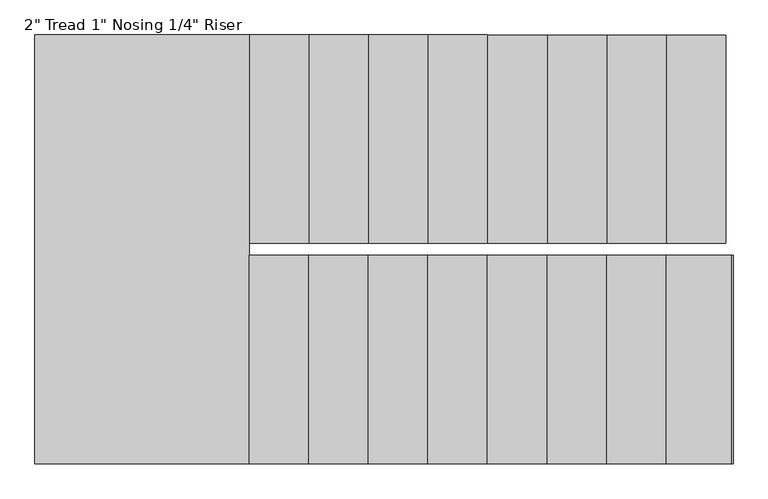
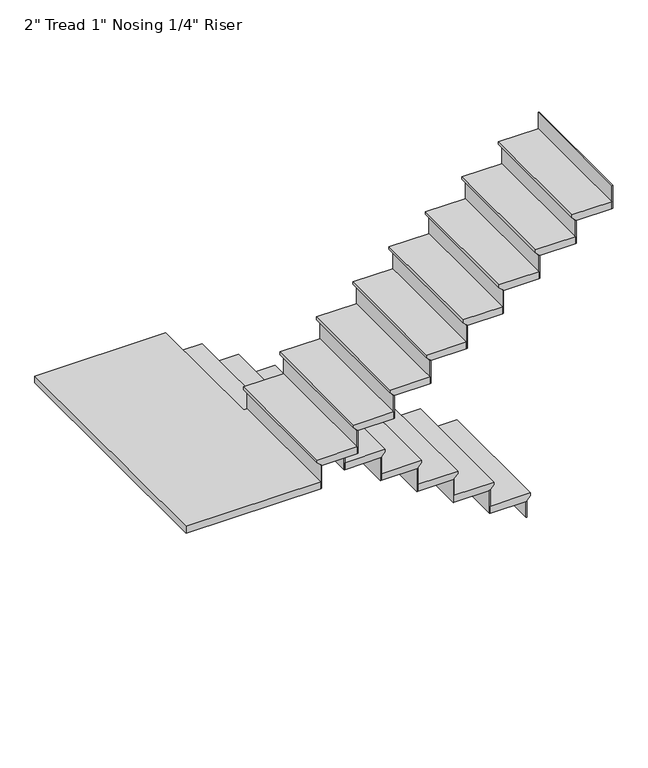
"""IFC4 building model written with IfcOpenShell, lengths in millimetres: stair flight geometry."""

from ifc_helpers import new_model, si_unit, origin, place, context, project, spatial, faceted_brep, source, transform, mapped, element, save


def stair_flight_f55dda53(model_context):
    return source(origin(), model_context, "Body", "Brep", [
        faceted_brep([(-2748.0012202, 5930.6309003, 15390.2833333), (-2748.0012202, 5930.6309003, 15409.3333333), (-2748.0012202, 5041.6309003, 15409.3333333), (-2748.0012202, 5041.6309003, 15390.2833333), (-2773.4012202, 5930.6309003, 15364.8833333), (-2773.4012202, 5041.6309003, 15364.8833333), (-3027.4012202, 5930.6309003, 15409.3333333), (-3027.4012202, 5041.6309003, 15409.3333333), (-2773.4012202, 5041.6309003, 15358.5333333), (-3027.4012202, 5041.6309003, 15358.5333333), (-3027.4012202, 5930.6309003, 15358.5333333), (-2773.4012202, 5930.6309003, 15358.5333333)], [[[0, 1, 2, 3]], [[4, 0, 3, 5]], [[2, 1, 6, 7]], [[8, 9, 10, 11]], [[2, 7, 9, 8, 5, 3]], [[8, 11, 4, 5]], [[6, 1, 0, 4, 11, 10]], [[7, 6, 10, 9]]]),
        faceted_brep([(-2773.4012202, 5930.6309003, 15358.5333333), (-2773.4012202, 5930.6309003, 15240.0), (-2779.7512202, 5930.6309003, 15240.0), (-2779.7512202, 5930.6309003, 15358.5333333), (-2773.4012202, 5041.6309003, 15358.5333333), (-2779.7512202, 5041.6309003, 15358.5333333), (-2779.7512202, 5041.6309003, 15240.0), (-2773.4012202, 5041.6309003, 15240.0)], [[[0, 1, 2, 3]], [[4, 5, 6, 7]], [[1, 0, 4, 7]], [[2, 1, 7, 6]], [[3, 2, 6, 5]], [[0, 3, 5, 4]]]),
        faceted_brep([(-3027.4012202, 5930.6309003, 15527.8666667), (-3027.4012202, 5930.6309003, 15358.5333333), (-3033.7512202, 5930.6309003, 15358.5333333), (-3033.7512202, 5930.6309003, 15527.8666667), (-3027.4012202, 5041.6309003, 15527.8666667), (-3033.7512202, 5041.6309003, 15527.8666667), (-3033.7512202, 5041.6309003, 15358.5333333), (-3027.4012202, 5041.6309003, 15358.5333333)], [[[0, 1, 2, 3]], [[4, 5, 6, 7]], [[1, 0, 4, 7]], [[2, 1, 7, 6]], [[3, 2, 6, 5]], [[0, 3, 5, 4]]]),
        faceted_brep([(-3002.0012202, 5041.6309003, 15578.6666667), (-3002.0012202, 5930.6309003, 15578.6666667), (-3281.4012202, 5930.6309003, 15578.6666667), (-3281.4012202, 5041.6309003, 15578.6666667), (-3027.4012202, 5041.6309003, 15527.8666667), (-3281.4012202, 5041.6309003, 15527.8666667), (-3281.4012202, 5930.6309003, 15527.8666667), (-3027.4012202, 5930.6309003, 15527.8666667), (-3027.4012202, 5041.6309003, 15534.2166667), (-3002.0012202, 5041.6309003, 15559.6166667), (-3027.4012202, 5930.6309003, 15534.2166667), (-3002.0012202, 5930.6309003, 15559.6166667)], [[[0, 1, 2, 3]], [[4, 5, 6, 7]], [[0, 3, 5, 4, 8, 9]], [[4, 7, 10, 8]], [[2, 1, 11, 10, 7, 6]], [[3, 2, 6, 5]], [[11, 1, 0, 9]], [[10, 11, 9, 8]]]),
        faceted_brep([(-3281.4012202, 5930.6309003, 15697.2), (-3281.4012202, 5930.6309003, 15527.8666667), (-3287.7512202, 5930.6309003, 15527.8666667), (-3287.7512202, 5930.6309003, 15697.2), (-3281.4012202, 5041.6309003, 15697.2), (-3287.7512202, 5041.6309003, 15697.2), (-3287.7512202, 5041.6309003, 15527.8666667), (-3281.4012202, 5041.6309003, 15527.8666667)], [[[0, 1, 2, 3]], [[4, 5, 6, 7]], [[1, 0, 4, 7]], [[2, 1, 7, 6]], [[3, 2, 6, 5]], [[0, 3, 5, 4]]]),
        faceted_brep([(-3256.0012202, 5041.6309003, 15748.0), (-3256.0012202, 5930.6309003, 15748.0), (-3535.4012202, 5930.6309003, 15748.0), (-3535.4012202, 5041.6309003, 15748.0), (-3281.4012202, 5041.6309003, 15697.2), (-3535.4012202, 5041.6309003, 15697.2), (-3535.4012202, 5930.6309003, 15697.2), (-3281.4012202, 5930.6309003, 15697.2), (-3281.4012202, 5041.6309003, 15703.55), (-3256.0012202, 5041.6309003, 15728.95), (-3281.4012202, 5930.6309003, 15703.55), (-3256.0012202, 5930.6309003, 15728.95)], [[[0, 1, 2, 3]], [[4, 5, 6, 7]], [[0, 3, 5, 4, 8, 9]], [[4, 7, 10, 8]], [[2, 1, 11, 10, 7, 6]], [[3, 2, 6, 5]], [[11, 1, 0, 9]], [[10, 11, 9, 8]]]),
        faceted_brep([(-3535.4012202, 5930.6309003, 15866.5333333), (-3535.4012202, 5930.6309003, 15697.2), (-3541.7512202, 5930.6309003, 15697.2), (-3541.7512202, 5930.6309003, 15866.5333333), (-3535.4012202, 5041.6309003, 15866.5333333), (-3541.7512202, 5041.6309003, 15866.5333333), (-3541.7512202, 5041.6309003, 15697.2), (-3535.4012202, 5041.6309003, 15697.2)], [[[0, 1, 2, 3]], [[4, 5, 6, 7]], [[1, 0, 4, 7]], [[2, 1, 7, 6]], [[3, 2, 6, 5]], [[0, 3, 5, 4]]]),
        faceted_brep([(-3510.0012202, 5041.6309003, 15917.3333333), (-3510.0012202, 5930.6309003, 15917.3333333), (-3789.4012202, 5930.6309003, 15917.3333333), (-3789.4012202, 5041.6309003, 15917.3333333), (-3535.4012202, 5041.6309003, 15866.5333333), (-3789.4012202, 5041.6309003, 15866.5333333), (-3789.4012202, 5930.6309003, 15866.5333333), (-3535.4012202, 5930.6309003, 15866.5333333), (-3535.4012202, 5041.6309003, 15872.8833333), (-3510.0012202, 5041.6309003, 15898.2833333), (-3535.4012202, 5930.6309003, 15872.8833333), (-3510.0012202, 5930.6309003, 15898.2833333)], [[[0, 1, 2, 3]], [[4, 5, 6, 7]], [[0, 3, 5, 4, 8, 9]], [[4, 7, 10, 8]], [[2, 1, 11, 10, 7, 6]], [[3, 2, 6, 5]], [[11, 1, 0, 9]], [[10, 11, 9, 8]]]),
        faceted_brep([(-3789.4012202, 5930.6309003, 16035.8666667), (-3789.4012202, 5930.6309003, 15866.5333333), (-3795.7512202, 5930.6309003, 15866.5333333), (-3795.7512202, 5930.6309003, 16035.8666667), (-3789.4012202, 5041.6309003, 16035.8666667), (-3795.7512202, 5041.6309003, 16035.8666667), (-3795.7512202, 5041.6309003, 15866.5333333), (-3789.4012202, 5041.6309003, 15866.5333333)], [[[0, 1, 2, 3]], [[4, 5, 6, 7]], [[1, 0, 4, 7]], [[2, 1, 7, 6]], [[3, 2, 6, 5]], [[0, 3, 5, 4]]]),
        faceted_brep([(-3764.0012202, 5041.6309003, 16086.6666667), (-3764.0012202, 5930.6309003, 16086.6666667), (-4043.4012202, 5930.6309003, 16086.6666667), (-4043.4012202, 5041.6309003, 16086.6666667), (-3789.4012202, 5041.6309003, 16035.8666667), (-4043.4012202, 5041.6309003, 16035.8666667), (-4043.4012202, 5930.6309003, 16035.8666667), (-3789.4012202, 5930.6309003, 16035.8666667), (-3789.4012202, 5041.6309003, 16042.2166667), (-3764.0012202, 5041.6309003, 16067.6166667), (-3789.4012202, 5930.6309003, 16042.2166667), (-3764.0012202, 5930.6309003, 16067.6166667)], [[[0, 1, 2, 3]], [[4, 5, 6, 7]], [[0, 3, 5, 4, 8, 9]], [[4, 7, 10, 8]], [[2, 1, 11, 10, 7, 6]], [[3, 2, 6, 5]], [[11, 1, 0, 9]], [[10, 11, 9, 8]]]),
        faceted_brep([(-4043.4012202, 5930.6309003, 16205.2), (-4043.4012202, 5930.6309003, 16035.8666667), (-4049.7512202, 5930.6309003, 16035.8666667), (-4049.7512202, 5930.6309003, 16205.2), (-4043.4012202, 5041.6309003, 16205.2), (-4049.7512202, 5041.6309003, 16205.2), (-4049.7512202, 5041.6309003, 16035.8666667), (-4043.4012202, 5041.6309003, 16035.8666667)], [[[0, 1, 2, 3]], [[4, 5, 6, 7]], [[1, 0, 4, 7]], [[2, 1, 7, 6]], [[3, 2, 6, 5]], [[0, 3, 5, 4]]]),
        faceted_brep([(-4018.0012202, 5041.6309003, 16256.0), (-4018.0012202, 5930.6309003, 16256.0), (-4297.4012202, 5930.6309003, 16256.0), (-4297.4012202, 5041.6309003, 16256.0), (-4043.4012202, 5041.6309003, 16205.2), (-4297.4012202, 5041.6309003, 16205.2), (-4297.4012202, 5930.6309003, 16205.2), (-4043.4012202, 5930.6309003, 16205.2), (-4043.4012202, 5041.6309003, 16211.55), (-4018.0012202, 5041.6309003, 16236.95), (-4043.4012202, 5930.6309003, 16211.55), (-4018.0012202, 5930.6309003, 16236.95)], [[[0, 1, 2, 3]], [[4, 5, 6, 7]], [[0, 3, 5, 4, 8, 9]], [[4, 7, 10, 8]], [[2, 1, 11, 10, 7, 6]], [[3, 2, 6, 5]], [[11, 1, 0, 9]], [[10, 11, 9, 8]]]),
        faceted_brep([(-4297.4012202, 5930.6309003, 16374.5333333), (-4297.4012202, 5930.6309003, 16205.2), (-4303.7512202, 5930.6309003, 16205.2), (-4303.7512202, 5930.6309003, 16374.5333333), (-4297.4012202, 5041.6309003, 16374.5333333), (-4303.7512202, 5041.6309003, 16374.5333333), (-4303.7512202, 5041.6309003, 16205.2), (-4297.4012202, 5041.6309003, 16205.2)], [[[0, 1, 2, 3]], [[4, 5, 6, 7]], [[1, 0, 4, 7]], [[2, 1, 7, 6]], [[3, 2, 6, 5]], [[0, 3, 5, 4]]]),
        faceted_brep([(-4272.0012202, 5041.6309003, 16425.3333333), (-4272.0012202, 5930.6309003, 16425.3333333), (-4551.4012202, 5930.6309003, 16425.3333333), (-4551.4012202, 5041.6309003, 16425.3333333), (-4297.4012202, 5041.6309003, 16374.5333333), (-4551.4012202, 5041.6309003, 16374.5333333), (-4551.4012202, 5930.6309003, 16374.5333333), (-4297.4012202, 5930.6309003, 16374.5333333), (-4297.4012202, 5041.6309003, 16380.8833333), (-4272.0012202, 5041.6309003, 16406.2833333), (-4297.4012202, 5930.6309003, 16380.8833333), (-4272.0012202, 5930.6309003, 16406.2833333)], [[[0, 1, 2, 3]], [[4, 5, 6, 7]], [[0, 3, 5, 4, 8, 9]], [[4, 7, 10, 8]], [[2, 1, 11, 10, 7, 6]], [[3, 2, 6, 5]], [[11, 1, 0, 9]], [[10, 11, 9, 8]]]),
        faceted_brep([(-4551.4012202, 5930.6309003, 16543.8666667), (-4551.4012202, 5930.6309003, 16374.5333333), (-4557.7512202, 5930.6309003, 16374.5333333), (-4557.7512202, 5930.6309003, 16543.8666667), (-4551.4012202, 5041.6309003, 16543.8666667), (-4557.7512202, 5041.6309003, 16543.8666667), (-4557.7512202, 5041.6309003, 16374.5333333), (-4551.4012202, 5041.6309003, 16374.5333333)], [[[0, 1, 2, 3]], [[4, 5, 6, 7]], [[1, 0, 4, 7]], [[2, 1, 7, 6]], [[3, 2, 6, 5]], [[0, 3, 5, 4]]]),
        faceted_brep([(-4526.0012202, 5041.6309003, 16594.6666667), (-4526.0012202, 5930.6309003, 16594.6666667), (-4805.4012202, 5930.6309003, 16594.6666667), (-4805.4012202, 5041.6309003, 16594.6666667), (-4551.4012202, 5041.6309003, 16543.8666667), (-4805.4012202, 5041.6309003, 16543.8666667), (-4805.4012202, 5930.6309003, 16543.8666667), (-4551.4012202, 5930.6309003, 16543.8666667), (-4551.4012202, 5041.6309003, 16550.2166667), (-4526.0012202, 5041.6309003, 16575.6166667), (-4551.4012202, 5930.6309003, 16550.2166667), (-4526.0012202, 5930.6309003, 16575.6166667)], [[[0, 1, 2, 3]], [[4, 5, 6, 7]], [[0, 3, 5, 4, 8, 9]], [[4, 7, 10, 8]], [[2, 1, 11, 10, 7, 6]], [[3, 2, 6, 5]], [[11, 1, 0, 9]], [[10, 11, 9, 8]]]),
        faceted_brep([(-4805.4012202, 5930.6309003, 16713.2), (-4805.4012202, 5930.6309003, 16543.8666667), (-4811.7512202, 5930.6309003, 16543.8666667), (-4811.7512202, 5930.6309003, 16713.2), (-4805.4012202, 5041.6309003, 16713.2), (-4811.7512202, 5041.6309003, 16713.2), (-4811.7512202, 5041.6309003, 16543.8666667), (-4805.4012202, 5041.6309003, 16543.8666667)], [[[0, 1, 2, 3]], [[4, 5, 6, 7]], [[1, 0, 4, 7]], [[2, 1, 7, 6]], [[3, 2, 6, 5]], [[0, 3, 5, 4]]]),
        faceted_brep([(-4754.6012202, 4990.8309003, 16764.0), (-4780.0012202, 4990.8309003, 16764.0), (-4780.0012202, 5930.6309003, 16764.0), (-5694.4012202, 5930.6309003, 16764.0), (-5694.4012202, 4101.8309003, 16764.0), (-4754.6012202, 4101.8309003, 16764.0), (-4780.0012202, 4990.8309003, 16713.2), (-4754.6012202, 4990.8309003, 16713.2), (-4754.6012202, 4101.8309003, 16713.2), (-5694.4012202, 4101.8309003, 16713.2), (-5694.4012202, 5930.6309003, 16713.2), (-4805.4012202, 5930.6309003, 16713.2), (-4805.4012202, 5041.6309003, 16713.2), (-4780.0012202, 5041.6309003, 16713.2), (-4780.0012202, 5041.6309003, 16744.95), (-4780.0012202, 5930.6309003, 16744.95), (-4805.4012202, 5041.6309003, 16719.55), (-4805.4012202, 5930.6309003, 16719.55)], [[[0, 1, 2, 3, 4, 5]], [[6, 7, 8, 9, 10, 11, 12, 13]], [[1, 0, 7, 6]], [[2, 1, 6, 13, 14, 15]], [[13, 12, 16, 14]], [[12, 11, 17, 16]], [[3, 2, 15, 17, 11, 10]], [[4, 3, 10, 9]], [[5, 4, 9, 8]], [[0, 5, 8, 7]], [[17, 15, 14, 16]]]),
        faceted_brep([(-4754.6012202, 4101.8309003, 16882.5333333), (-4754.6012202, 4101.8309003, 16713.2), (-4748.2512202, 4101.8309003, 16713.2), (-4748.2512202, 4101.8309003, 16882.5333333), (-4754.6012202, 4990.8309003, 16882.5333333), (-4748.2512202, 4990.8309003, 16882.5333333), (-4748.2512202, 4990.8309003, 16713.2), (-4754.6012202, 4990.8309003, 16713.2)], [[[0, 1, 2, 3]], [[4, 5, 6, 7]], [[1, 0, 4, 7]], [[2, 1, 7, 6]], [[3, 2, 6, 5]], [[0, 3, 5, 4]]]),
        faceted_brep([(-4780.0012202, 4990.8309003, 16933.3333333), (-4780.0012202, 4101.8309003, 16933.3333333), (-4500.6012202, 4101.8309003, 16933.3333333), (-4500.6012202, 4990.8309003, 16933.3333333), (-4754.6012202, 4990.8309003, 16882.5333333), (-4500.6012202, 4990.8309003, 16882.5333333), (-4500.6012202, 4101.8309003, 16882.5333333), (-4754.6012202, 4101.8309003, 16882.5333333), (-4754.6012202, 4990.8309003, 16888.8833333), (-4780.0012202, 4990.8309003, 16914.2833333), (-4754.6012202, 4101.8309003, 16888.8833333), (-4780.0012202, 4101.8309003, 16914.2833333)], [[[0, 1, 2, 3]], [[4, 5, 6, 7]], [[0, 3, 5, 4, 8, 9]], [[4, 7, 10, 8]], [[2, 1, 11, 10, 7, 6]], [[3, 2, 6, 5]], [[11, 1, 0, 9]], [[10, 11, 9, 8]]]),
        faceted_brep([(-4500.6012202, 4101.8309003, 17051.8666667), (-4500.6012202, 4101.8309003, 16882.5333333), (-4494.2512202, 4101.8309003, 16882.5333333), (-4494.2512202, 4101.8309003, 17051.8666667), (-4500.6012202, 4990.8309003, 17051.8666667), (-4494.2512202, 4990.8309003, 17051.8666667), (-4494.2512202, 4990.8309003, 16882.5333333), (-4500.6012202, 4990.8309003, 16882.5333333)], [[[0, 1, 2, 3]], [[4, 5, 6, 7]], [[1, 0, 4, 7]], [[2, 1, 7, 6]], [[3, 2, 6, 5]], [[0, 3, 5, 4]]]),
        faceted_brep([(-4526.0012202, 4990.8309003, 17102.6666667), (-4526.0012202, 4101.8309003, 17102.6666667), (-4246.6012202, 4101.8309003, 17102.6666667), (-4246.6012202, 4990.8309003, 17102.6666667), (-4500.6012202, 4990.8309003, 17051.8666667), (-4246.6012202, 4990.8309003, 17051.8666667), (-4246.6012202, 4101.8309003, 17051.8666667), (-4500.6012202, 4101.8309003, 17051.8666667), (-4500.6012202, 4990.8309003, 17058.2166667), (-4526.0012202, 4990.8309003, 17083.6166667), (-4500.6012202, 4101.8309003, 17058.2166667), (-4526.0012202, 4101.8309003, 17083.6166667)], [[[0, 1, 2, 3]], [[4, 5, 6, 7]], [[0, 3, 5, 4, 8, 9]], [[4, 7, 10, 8]], [[2, 1, 11, 10, 7, 6]], [[3, 2, 6, 5]], [[11, 1, 0, 9]], [[10, 11, 9, 8]]]),
        faceted_brep([(-4246.6012202, 4101.8309003, 17221.2), (-4246.6012202, 4101.8309003, 17051.8666667), (-4240.2512202, 4101.8309003, 17051.8666667), (-4240.2512202, 4101.8309003, 17221.2), (-4246.6012202, 4990.8309003, 17221.2), (-4240.2512202, 4990.8309003, 17221.2), (-4240.2512202, 4990.8309003, 17051.8666667), (-4246.6012202, 4990.8309003, 17051.8666667)], [[[0, 1, 2, 3]], [[4, 5, 6, 7]], [[1, 0, 4, 7]], [[2, 1, 7, 6]], [[3, 2, 6, 5]], [[0, 3, 5, 4]]]),
        faceted_brep([(-4272.0012202, 4990.8309003, 17272.0), (-4272.0012202, 4101.8309003, 17272.0), (-3992.6012202, 4101.8309003, 17272.0), (-3992.6012202, 4990.8309003, 17272.0), (-4246.6012202, 4990.8309003, 17221.2), (-3992.6012202, 4990.8309003, 17221.2), (-3992.6012202, 4101.8309003, 17221.2), (-4246.6012202, 4101.8309003, 17221.2), (-4246.6012202, 4990.8309003, 17227.55), (-4272.0012202, 4990.8309003, 17252.95), (-4246.6012202, 4101.8309003, 17227.55), (-4272.0012202, 4101.8309003, 17252.95)], [[[0, 1, 2, 3]], [[4, 5, 6, 7]], [[0, 3, 5, 4, 8, 9]], [[4, 7, 10, 8]], [[2, 1, 11, 10, 7, 6]], [[3, 2, 6, 5]], [[11, 1, 0, 9]], [[10, 11, 9, 8]]]),
        faceted_brep([(-3992.6012202, 4101.8309003, 17390.5333333), (-3992.6012202, 4101.8309003, 17221.2), (-3986.2512202, 4101.8309003, 17221.2), (-3986.2512202, 4101.8309003, 17390.5333333), (-3992.6012202, 4990.8309003, 17390.5333333), (-3986.2512202, 4990.8309003, 17390.5333333), (-3986.2512202, 4990.8309003, 17221.2), (-3992.6012202, 4990.8309003, 17221.2)], [[[0, 1, 2, 3]], [[4, 5, 6, 7]], [[1, 0, 4, 7]], [[2, 1, 7, 6]], [[3, 2, 6, 5]], [[0, 3, 5, 4]]]),
        faceted_brep([(-4018.0012202, 4990.8309003, 17441.3333333), (-4018.0012202, 4101.8309003, 17441.3333333), (-3738.6012202, 4101.8309003, 17441.3333333), (-3738.6012202, 4990.8309003, 17441.3333333), (-3992.6012202, 4990.8309003, 17390.5333333), (-3738.6012202, 4990.8309003, 17390.5333333), (-3738.6012202, 4101.8309003, 17390.5333333), (-3992.6012202, 4101.8309003, 17390.5333333), (-3992.6012202, 4990.8309003, 17396.8833333), (-4018.0012202, 4990.8309003, 17422.2833333), (-3992.6012202, 4101.8309003, 17396.8833333), (-4018.0012202, 4101.8309003, 17422.2833333)], [[[0, 1, 2, 3]], [[4, 5, 6, 7]], [[0, 3, 5, 4, 8, 9]], [[4, 7, 10, 8]], [[2, 1, 11, 10, 7, 6]], [[3, 2, 6, 5]], [[11, 1, 0, 9]], [[10, 11, 9, 8]]]),
        faceted_brep([(-3738.6012202, 4101.8309003, 17559.8666667), (-3738.6012202, 4101.8309003, 17390.5333333), (-3732.2512202, 4101.8309003, 17390.5333333), (-3732.2512202, 4101.8309003, 17559.8666667), (-3738.6012202, 4990.8309003, 17559.8666667), (-3732.2512202, 4990.8309003, 17559.8666667), (-3732.2512202, 4990.8309003, 17390.5333333), (-3738.6012202, 4990.8309003, 17390.5333333)], [[[0, 1, 2, 3]], [[4, 5, 6, 7]], [[1, 0, 4, 7]], [[2, 1, 7, 6]], [[3, 2, 6, 5]], [[0, 3, 5, 4]]]),
        faceted_brep([(-3764.0012202, 4990.8309003, 17610.6666667), (-3764.0012202, 4101.8309003, 17610.6666667), (-3484.6012202, 4101.8309003, 17610.6666667), (-3484.6012202, 4990.8309003, 17610.6666667), (-3738.6012202, 4990.8309003, 17559.8666667), (-3484.6012202, 4990.8309003, 17559.8666667), (-3484.6012202, 4101.8309003, 17559.8666667), (-3738.6012202, 4101.8309003, 17559.8666667), (-3738.6012202, 4990.8309003, 17566.2166667), (-3764.0012202, 4990.8309003, 17591.6166667), (-3738.6012202, 4101.8309003, 17566.2166667), (-3764.0012202, 4101.8309003, 17591.6166667)], [[[0, 1, 2, 3]], [[4, 5, 6, 7]], [[0, 3, 5, 4, 8, 9]], [[4, 7, 10, 8]], [[2, 1, 11, 10, 7, 6]], [[3, 2, 6, 5]], [[11, 1, 0, 9]], [[10, 11, 9, 8]]]),
        faceted_brep([(-3484.6012202, 4101.8309003, 17729.2), (-3484.6012202, 4101.8309003, 17559.8666667), (-3478.2512202, 4101.8309003, 17559.8666667), (-3478.2512202, 4101.8309003, 17729.2), (-3484.6012202, 4990.8309003, 17729.2), (-3478.2512202, 4990.8309003, 17729.2), (-3478.2512202, 4990.8309003, 17559.8666667), (-3484.6012202, 4990.8309003, 17559.8666667)], [[[0, 1, 2, 3]], [[4, 5, 6, 7]], [[1, 0, 4, 7]], [[2, 1, 7, 6]], [[3, 2, 6, 5]], [[0, 3, 5, 4]]]),
        faceted_brep([(-3510.0012202, 4990.8309003, 17780.0), (-3510.0012202, 4101.8309003, 17780.0), (-3230.6012202, 4101.8309003, 17780.0), (-3230.6012202, 4990.8309003, 17780.0), (-3484.6012202, 4990.8309003, 17729.2), (-3230.6012202, 4990.8309003, 17729.2), (-3230.6012202, 4101.8309003, 17729.2), (-3484.6012202, 4101.8309003, 17729.2), (-3484.6012202, 4990.8309003, 17735.55), (-3510.0012202, 4990.8309003, 17760.95), (-3484.6012202, 4101.8309003, 17735.55), (-3510.0012202, 4101.8309003, 17760.95)], [[[0, 1, 2, 3]], [[4, 5, 6, 7]], [[0, 3, 5, 4, 8, 9]], [[4, 7, 10, 8]], [[2, 1, 11, 10, 7, 6]], [[3, 2, 6, 5]], [[11, 1, 0, 9]], [[10, 11, 9, 8]]]),
        faceted_brep([(-3230.6012202, 4101.8309003, 17898.5333333), (-3230.6012202, 4101.8309003, 17729.2), (-3224.2512202, 4101.8309003, 17729.2), (-3224.2512202, 4101.8309003, 17898.5333333), (-3230.6012202, 4990.8309003, 17898.5333333), (-3224.2512202, 4990.8309003, 17898.5333333), (-3224.2512202, 4990.8309003, 17729.2), (-3230.6012202, 4990.8309003, 17729.2)], [[[0, 1, 2, 3]], [[4, 5, 6, 7]], [[1, 0, 4, 7]], [[2, 1, 7, 6]], [[3, 2, 6, 5]], [[0, 3, 5, 4]]]),
        faceted_brep([(-3256.0012202, 4990.8309003, 17949.3333333), (-3256.0012202, 4101.8309003, 17949.3333333), (-2976.6012202, 4101.8309003, 17949.3333333), (-2976.6012202, 4990.8309003, 17949.3333333), (-3230.6012202, 4990.8309003, 17898.5333333), (-2976.6012202, 4990.8309003, 17898.5333333), (-2976.6012202, 4101.8309003, 17898.5333333), (-3230.6012202, 4101.8309003, 17898.5333333), (-3230.6012202, 4990.8309003, 17904.8833333), (-3256.0012202, 4990.8309003, 17930.2833333), (-3230.6012202, 4101.8309003, 17904.8833333), (-3256.0012202, 4101.8309003, 17930.2833333)], [[[0, 1, 2, 3]], [[4, 5, 6, 7]], [[0, 3, 5, 4, 8, 9]], [[4, 7, 10, 8]], [[2, 1, 11, 10, 7, 6]], [[3, 2, 6, 5]], [[11, 1, 0, 9]], [[10, 11, 9, 8]]]),
        faceted_brep([(-2976.6012202, 4101.8309003, 18067.8666667), (-2976.6012202, 4101.8309003, 17898.5333333), (-2970.2512202, 4101.8309003, 17898.5333333), (-2970.2512202, 4101.8309003, 18067.8666667), (-2976.6012202, 4990.8309003, 18067.8666667), (-2970.2512202, 4990.8309003, 18067.8666667), (-2970.2512202, 4990.8309003, 17898.5333333), (-2976.6012202, 4990.8309003, 17898.5333333)], [[[0, 1, 2, 3]], [[4, 5, 6, 7]], [[1, 0, 4, 7]], [[2, 1, 7, 6]], [[3, 2, 6, 5]], [[0, 3, 5, 4]]]),
        faceted_brep([(-2722.6012202, 4101.8309003, 18237.2), (-2722.6012202, 4101.8309003, 18067.8666667), (-2716.2512202, 4101.8309003, 18067.8666667), (-2716.2512202, 4101.8309003, 18237.2), (-2722.6012202, 4990.8309003, 18237.2), (-2716.2512202, 4990.8309003, 18237.2), (-2716.2512202, 4990.8309003, 18067.8666667), (-2722.6012202, 4990.8309003, 18067.8666667)], [[[0, 1, 2, 3]], [[4, 5, 6, 7]], [[1, 0, 4, 7]], [[2, 1, 7, 6]], [[3, 2, 6, 5]], [[0, 3, 5, 4]]]),
        faceted_brep([(-3002.0012202, 4990.8309003, 18118.6666667), (-3002.0012202, 4101.8309003, 18118.6666667), (-2722.6012202, 4101.8309003, 18118.6666667), (-2722.6012202, 4990.8309003, 18118.6666667), (-2976.6012202, 4990.8309003, 18067.8666667), (-2722.6012202, 4990.8309003, 18067.8666667), (-2722.6012202, 4101.8309003, 18067.8666667), (-2976.6012202, 4101.8309003, 18067.8666667), (-2976.6012202, 4990.8309003, 18074.2166667), (-3002.0012202, 4990.8309003, 18099.6166667), (-2976.6012202, 4101.8309003, 18074.2166667), (-3002.0012202, 4101.8309003, 18099.6166667)], [[[0, 1, 2, 3]], [[4, 5, 6, 7]], [[0, 3, 5, 4, 8, 9]], [[4, 7, 10, 8]], [[2, 1, 11, 10, 7, 6]], [[3, 2, 6, 5]], [[11, 1, 0, 9]], [[10, 11, 9, 8]]]),
    ])


if __name__ == "__main__":
    model = new_model("IFC4")
    model_context = context("Model", 3, world=origin())
    ifc_project = project(units=[si_unit("LENGTHUNIT", "METRE", prefix="MILLI")], contexts=[model_context])
    site = spatial("IfcSite", under=ifc_project)
    building = spatial("IfcBuilding", under=site)
    placement = place(None, origin())
    stair_flight_shape = stair_flight_f55dda53(model_context)
    element("IfcStairFlight", 1, ObjectType="2\" Tread 1\" Nosing 1/4\" Riser", at=placement, inside=building, context=model_context, shape_type="MappedRepresentation", body=[
        mapped(stair_flight_shape, transform((0.0, 0.0, 0.0), x_axis=(1.0, 0.0, 0.0), y_axis=(0.0, 1.0, 0.0), z_axis=(0.0, 0.0, 1.0))),
    ])
    save(model, "model.ifc")
